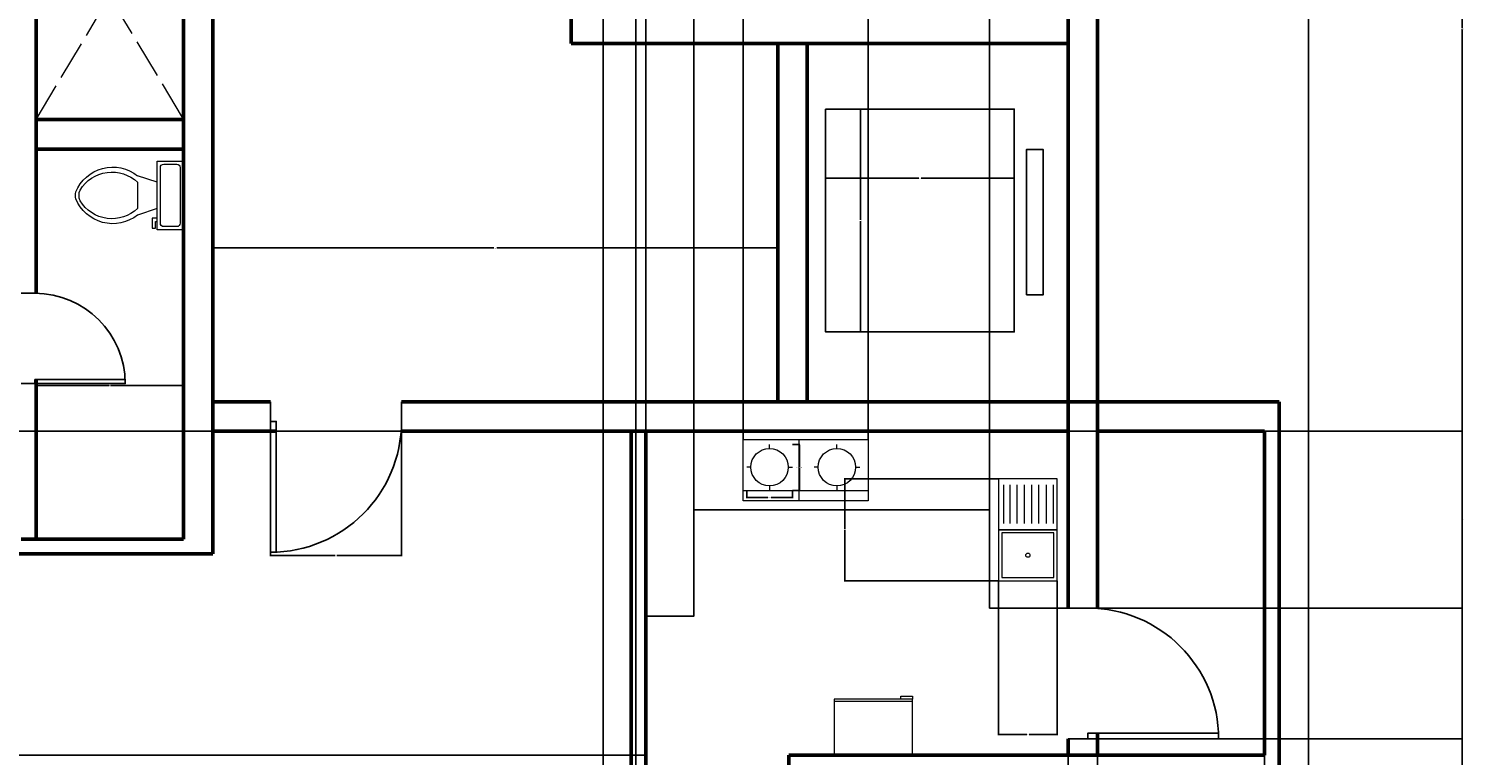
# Model space of a CAD drawing. Units: inches. Extents: x 2032 to 3981, y 840 to 2177.
# Tile 3 of 6: x 2286 to 2725, y 1132 to 1354. Entities that reach past the tile are written whole.
import ezdxf

# ---------------------------------------------------------------- set-up
doc = ezdxf.new("R2010")
doc.units = ezdxf.units.IN
doc.linetypes.add('ACAD_ISO02W100', pattern=[15, 12, -3])
for name, color, linetype, lineweight in [('A-ANNO-DIMS', 2, 'Continuous', 18), ('A-DOOR', 3, 'Continuous', 25), ('A-EQPM', 8, 'Continuous', 18), ('A-FLOR-CASE', 32, 'Continuous', 25), ('A-FLOR-EVTR', 8, 'Continuous', 25), ('A-FLOR-FIXT', 9, 'Continuous', 18), ('A-FLOR-OPEN', 8, 'ACAD_ISO02W100', 13), ('A-WALL', 7, 'Continuous', 50)]:
    doc.layers.add(name, color=color, linetype=linetype, lineweight=lineweight)
doc.styles.get("Standard").update_dxf_attribs({"font": 'arial.ttf'})
doc.dimstyles.get("Standard").update_dxf_attribs({"dimtxt": 0.18, "dimasz": 0.18, "dimexe": 0.18, "dimexo": 0.0625, "dimgap": 0.09, "dimtad": 0, "dimtih": 1, "dimtoh": 1, "dimdec": 4, "dimzin": 0, "dimdsep": 46, "dimtxsty": 'Standard', "dimcen": 0.09, "dimadec": 0, "dimazin": 0, "dimtfac": 1, "dimtdec": 4, "dimtofl": 0, "dimtmove": 0, "dimatfit": 3, "dimfxl": 1, "dimtolj": 1, "dimtzin": 0, "dimarcsym": 0})

# ---------------------------------------------------------------- blocks, each defined once
blk = doc.blocks.new('*U2')
for p, q in [((0, 0), (0, -6)), ((40, 0), (40, -6))]:
    blk.add_line(p, q)
blk.add_lwpolyline([(0, 0), (0, 40), (1.75, 40), (1.75, 0)], close=True)
blk.add_arc((0, 0), 40, 0, 90)
blk = doc.blocks.new('*U4')
for p, q in [((9.5, -6), (9.5, -2)), ((-10, -8.5), (-8, -8.5)), ((-10, -9.5), (-10, -8.5)), ((-8, -8.5), (-8, -8)), ((-7, -8), (-7, -9.5)), ((-4, -8), (-6, -14)), ((4, -8), (6, -14)), ((-7, -9.5), (-10, -9.5)), ((4, -14), (-4, -14))]:
    blk.add_line(p, q)
blk.add_lwpolyline([(10.5, -8), (10.5, 0), (-10.5, 0), (-10.5, -8)], close=True)
for points in [[(-9.5, -2), (-9.5, -6)], [(8.5, -1), (-8.5, -1)], [(-8.5, -7), (8.5, -7)]]:
    blk.add_lwpolyline(points)
for centre, radius, start, end in [((-8.62, -1.88), 0.884, 81.8699, 188.1301), ((8.62, -1.88), 0.884, 351.8699, 98.1301), ((-8.62, -6.12), 0.884, 171.8699, 278.1301), ((8.62, -6.12), 0.884, 261.8699, 8.1301), ((3.52, -21.58), 12.17, 141.4691, 247.9714), ((4.2, -21.82), 11.33, 136.3677, 238.9468), ((-3.52, -21.58), 12.17, 292.0284, 38.5307), ((-4.2, -21.82), 11.33, 301.053, 43.6321), ((0, -27.88), 4, 245.7318, 294.2682), ((0, -29), 4, 254.8605, 285.1395)]:
    blk.add_arc(centre, radius, start, end)
blk = doc.blocks.new('COOKTOP-BURNER')
for p, q in [((6.97, 12.85), (6.97, 14.11)), ((1.25, 7.13), (0, 7.13)), ((12.69, 7.13), (13.97, 7.13)), ((6.97, 1.41), (6.97, 0))]:
    blk.add_line(p, q)
blk.add_circle((6.97, 7.13), 5.72)
blk = doc.blocks.new('*D12')
at = {"layer": 'A-ANNO-DIMS', "color": 0, "lineweight": -2, "transparency": 16777216}
for p, q in [((2519.81, 1226.93), (2522.05, 1226.93)), ((2521.87, 1226.75), (2521.87, 1220.06)), ((2521.87, 1213), (2521.87, 1219.7)), ((2519.81, 1212.82), (2522.05, 1212.82))]:
    blk.add_line(p, q, dxfattribs=at)
at = {"layer": 'A-ANNO-DIMS', "color": 0, "lineweight": 100, "transparency": 16777216}
for points in [[(2521.84, 1226.75), (2521.9, 1226.75), (2521.87, 1226.93)], [(2521.84, 1213), (2521.9, 1213), (2521.87, 1212.82)]]:
    blk.add_solid(points, dxfattribs=at)
at = {"layer": 'Defpoints', "color": 0, "lineweight": 100, "transparency": 16777216}
for p in [(2519.75, 1226.93), (2521.87, 1226.93), (2519.75, 1212.82)]:
    blk.add_point(p, dxfattribs=at)
at = {"layer": 'A-ANNO-DIMS', "color": 0, "transparency": 16777216, "insert": (2521.87, 1219.88), "char_height": 0.18, "attachment_point": 5}
blk.add_mtext('\\A1;BURNER 14 TYP.', dxfattribs=at)
blk = doc.blocks.new('*D13')
at = {"layer": 'A-ANNO-DIMS', "color": 0, "lineweight": -2, "transparency": 16777216}
for p, q in [((2505.78, 1212.76), (2505.78, 1210.53)), ((2505.96, 1210.71), (2512.25, 1210.71)), ((2519.57, 1210.71), (2513.29, 1210.71)), ((2519.75, 1212.76), (2519.75, 1210.53))]:
    blk.add_line(p, q, dxfattribs=at)
at = {"layer": 'A-ANNO-DIMS', "color": 0, "lineweight": 100, "transparency": 16777216}
for points in [[(2505.96, 1210.74), (2505.96, 1210.68), (2505.78, 1210.71)], [(2519.57, 1210.74), (2519.57, 1210.68), (2519.75, 1210.71)]]:
    blk.add_solid(points, dxfattribs=at)
at = {"layer": 'Defpoints', "color": 0, "lineweight": 100, "transparency": 16777216}
for p in [(2505.78, 1212.82), (2519.75, 1212.82), (2519.75, 1210.71)]:
    blk.add_point(p, dxfattribs=at)
at = {"layer": 'A-ANNO-DIMS', "color": 0, "transparency": 16777216, "insert": (2512.77, 1210.71), "char_height": 0.18, "attachment_point": 5}
blk.add_mtext('\\A1;14 TYP.', dxfattribs=at)
blk = doc.blocks.new('*D14')
at = {"layer": 'A-ANNO-DIMS', "color": 0, "lineweight": -2, "transparency": 16777216}
for p, q in [((2078.89, 1518.9), (2078.89, 840.08)), ((2677.35, 1476.9), (2677.35, 840.08)), ((2079.07, 840.26), (2377.73, 840.26)), ((2677.17, 840.26), (2378.52, 840.26))]:
    blk.add_line(p, q, dxfattribs=at)
at = {"layer": 'A-ANNO-DIMS', "color": 0, "lineweight": 100, "transparency": 16777216}
for points in [[(2079.07, 840.29), (2079.07, 840.23), (2078.89, 840.26)], [(2677.17, 840.29), (2677.17, 840.23), (2677.35, 840.26)]]:
    blk.add_solid(points, dxfattribs=at)
at = {"layer": 'Defpoints', "color": 0, "lineweight": 100, "transparency": 16777216}
for p in [(2078.89, 1518.96), (2677.35, 1476.96), (2677.35, 840.26)]:
    blk.add_point(p, dxfattribs=at)
at = {"layer": 'A-ANNO-DIMS', "color": 0, "transparency": 16777216, "insert": (2378.12, 840.26), "char_height": 0.18, "attachment_point": 5}
blk.add_mtext('\\A1;598.5', dxfattribs=at)
blk = doc.blocks.new('*D15')
at = {"layer": 'A-ANNO-DIMS', "color": 0, "lineweight": -2, "transparency": 16777216}
for p, q in [((2456.69, 1820.52), (2724.53, 1820.52)), ((2724.35, 1820.34), (2724.35, 1354.07)), ((2724.35, 887.44), (2724.35, 1353.71)), ((2476.27, 887.26), (2724.53, 887.26))]:
    blk.add_line(p, q, dxfattribs=at)
at = {"layer": 'A-ANNO-DIMS', "color": 0, "lineweight": 100, "transparency": 16777216}
for points in [[(2724.32, 1820.34), (2724.38, 1820.34), (2724.35, 1820.52)], [(2724.32, 887.44), (2724.38, 887.44), (2724.35, 887.26)]]:
    blk.add_solid(points, dxfattribs=at)
at = {"layer": 'Defpoints', "color": 0, "lineweight": 100, "transparency": 16777216}
for p in [(2456.63, 1820.52), (2476.21, 887.26), (2724.35, 887.26)]:
    blk.add_point(p, dxfattribs=at)
at = {"layer": 'A-ANNO-DIMS', "color": 0, "transparency": 16777216, "insert": (2724.35, 1353.89), "char_height": 0.18, "attachment_point": 5}
blk.add_mtext('\\A1;933.3', dxfattribs=at)
blk = doc.blocks.new('*D39')
at = {"layer": 'A-ANNO-DIMS', "color": 0, "lineweight": -2, "transparency": 16777216}
for p, q in [((2288.71, 1198.02), (2288.71, 1245.14)), ((2288.89, 1244.96), (2310.99, 1244.96)), ((2333.53, 1244.96), (2311.43, 1244.96)), ((2333.71, 1198.02), (2333.71, 1245.14))]:
    blk.add_line(p, q, dxfattribs=at)
at = {"layer": 'A-ANNO-DIMS', "color": 0, "lineweight": 100, "transparency": 16777216}
for points in [[(2288.89, 1244.99), (2288.89, 1244.93), (2288.71, 1244.96)], [(2333.53, 1244.99), (2333.53, 1244.93), (2333.71, 1244.96)]]:
    blk.add_solid(points, dxfattribs=at)
at = {"layer": 'Defpoints', "color": 0, "lineweight": 100, "transparency": 16777216}
for p in [(2333.71, 1244.96), (2288.71, 1197.96), (2333.71, 1197.96)]:
    blk.add_point(p, dxfattribs=at)
at = {"layer": 'A-ANNO-DIMS', "color": 0, "transparency": 16777216, "insert": (2311.21, 1244.96), "char_height": 0.18, "attachment_point": 5}
blk.add_mtext('\\A1;45', dxfattribs=at)
blk = doc.blocks.new('*D40')
at = {"layer": 'A-ANNO-DIMS', "color": 0, "lineweight": -2, "transparency": 16777216}
for p, q in [((2342.71, 1240.02), (2342.71, 1287.14)), ((2342.89, 1286.96), (2428.53, 1286.96)), ((2515.07, 1286.96), (2429.43, 1286.96)), ((2515.25, 1240.02), (2515.25, 1287.14))]:
    blk.add_line(p, q, dxfattribs=at)
at = {"layer": 'A-ANNO-DIMS', "color": 0, "lineweight": 100, "transparency": 16777216}
for points in [[(2342.89, 1286.99), (2342.89, 1286.93), (2342.71, 1286.96)], [(2515.07, 1286.99), (2515.07, 1286.93), (2515.25, 1286.96)]]:
    blk.add_solid(points, dxfattribs=at)
at = {"layer": 'Defpoints', "color": 0, "lineweight": 100, "transparency": 16777216}
for p in [(2515.25, 1286.96), (2342.71, 1239.96), (2515.25, 1239.96)]:
    blk.add_point(p, dxfattribs=at)
at = {"layer": 'A-ANNO-DIMS', "color": 0, "transparency": 16777216, "insert": (2428.98, 1286.96), "char_height": 0.18, "attachment_point": 5}
blk.add_mtext('\\A1;172.54', dxfattribs=at)
blk = doc.blocks.new('*D41')
at = {"layer": 'A-ANNO-DIMS', "color": 0, "lineweight": -2, "transparency": 16777216}
for p, q in [((2529.88, 1261.33), (2529.88, 1308.45)), ((2530.06, 1308.27), (2558.31, 1308.27)), ((2587.31, 1308.27), (2559.06, 1308.27)), ((2587.49, 1261.33), (2587.49, 1308.45))]:
    blk.add_line(p, q, dxfattribs=at)
at = {"layer": 'A-ANNO-DIMS', "color": 0, "lineweight": 100, "transparency": 16777216}
for points in [[(2530.06, 1308.3), (2530.06, 1308.24), (2529.88, 1308.27)], [(2587.31, 1308.3), (2587.31, 1308.24), (2587.49, 1308.27)]]:
    blk.add_solid(points, dxfattribs=at)
at = {"layer": 'Defpoints', "color": 0, "lineweight": 100, "transparency": 16777216}
for p in [(2587.49, 1308.27), (2529.88, 1261.27), (2587.49, 1261.27)]:
    blk.add_point(p, dxfattribs=at)
at = {"layer": 'A-ANNO-DIMS', "color": 0, "transparency": 16777216, "insert": (2558.68, 1308.27), "char_height": 0.18, "attachment_point": 5}
blk.add_mtext('\\A1;57.61', dxfattribs=at)
blk = doc.blocks.new('*D42')
at = {"layer": 'A-ANNO-DIMS', "color": 0, "lineweight": -2, "transparency": 16777216}
for p, q in [((2587.42, 1329.38), (2540.31, 1329.38)), ((2540.49, 1329.2), (2540.49, 1295.51)), ((2540.49, 1261.45), (2540.49, 1295.14)), ((2587.42, 1261.27), (2540.31, 1261.27))]:
    blk.add_line(p, q, dxfattribs=at)
at = {"layer": 'A-ANNO-DIMS', "color": 0, "lineweight": 100, "transparency": 16777216}
for points in [[(2540.46, 1329.2), (2540.52, 1329.2), (2540.49, 1329.38)], [(2540.46, 1261.45), (2540.52, 1261.45), (2540.49, 1261.27)]]:
    blk.add_solid(points, dxfattribs=at)
at = {"layer": 'Defpoints', "color": 0, "lineweight": 100, "transparency": 16777216}
for p in [(2540.49, 1329.38), (2587.49, 1329.38), (2587.49, 1261.27)]:
    blk.add_point(p, dxfattribs=at)
at = {"layer": 'A-ANNO-DIMS', "color": 0, "transparency": 16777216, "insert": (2540.49, 1295.33), "char_height": 0.18, "attachment_point": 5}
blk.add_mtext('\\A1;68.11', dxfattribs=at)
blk = doc.blocks.new('*D43')
at = {"layer": 'A-ANNO-DIMS', "color": 0, "lineweight": -2, "transparency": 16777216}
for p, q in [((2360.34, 1239.9), (2360.34, 1192.78)), ((2400.34, 1239.9), (2400.34, 1192.78)), ((2360.52, 1192.96), (2380.11, 1192.96)), ((2400.16, 1192.96), (2380.56, 1192.96))]:
    blk.add_line(p, q, dxfattribs=at)
at = {"layer": 'A-ANNO-DIMS', "color": 0, "lineweight": 100, "transparency": 16777216}
for points in [[(2360.52, 1192.99), (2360.52, 1192.93), (2360.34, 1192.96)], [(2400.16, 1192.99), (2400.16, 1192.93), (2400.34, 1192.96)]]:
    blk.add_solid(points, dxfattribs=at)
at = {"layer": 'Defpoints', "color": 0, "lineweight": 100, "transparency": 16777216}
for p in [(2360.34, 1239.96), (2400.34, 1239.96), (2360.34, 1192.96)]:
    blk.add_point(p, dxfattribs=at)
at = {"layer": 'A-ANNO-DIMS', "color": 0, "transparency": 16777216, "insert": (2380.34, 1192.96), "char_height": 0.18, "attachment_point": 5}
blk.add_mtext('\\A1;40', dxfattribs=at)
blk = doc.blocks.new('*D51')
at = {"layer": 'A-ANNO-DIMS', "color": 0, "lineweight": -2, "transparency": 16777216}
for p, q in [((2474.93, 1231.02), (2474.93, 1867.7)), ((2475.11, 1867.52), (2481.81, 1867.52)), ((2489.42, 1867.52), (2482.72, 1867.52)), ((2489.6, 1231.02), (2489.6, 1867.7))]:
    blk.add_line(p, q, dxfattribs=at)
at = {"layer": 'A-ANNO-DIMS', "color": 0, "lineweight": 100, "transparency": 16777216}
for points in [[(2475.11, 1867.55), (2475.11, 1867.49), (2474.93, 1867.52)], [(2489.42, 1867.55), (2489.42, 1867.49), (2489.6, 1867.52)]]:
    blk.add_solid(points, dxfattribs=at)
at = {"layer": 'Defpoints', "color": 0, "lineweight": 100, "transparency": 16777216}
for p in [(2489.6, 1867.52), (2474.93, 1230.96), (2489.6, 1230.96)]:
    blk.add_point(p, dxfattribs=at)
at = {"layer": 'A-ANNO-DIMS', "color": 0, "transparency": 16777216, "insert": (2482.27, 1867.52), "char_height": 0.18, "attachment_point": 5}
blk.add_mtext('\\A1;14.668', dxfattribs=at)
blk = doc.blocks.new('*D52')
at = {"layer": 'A-ANNO-DIMS', "color": 0, "lineweight": -2, "transparency": 16777216}
for p, q in [((2489.6, 1231.02), (2489.6, 1867.7)), ((2489.78, 1867.52), (2496.71, 1867.52)), ((2504.55, 1867.52), (2497.62, 1867.52)), ((2504.73, 1228.5), (2504.73, 1867.7))]:
    blk.add_line(p, q, dxfattribs=at)
at = {"layer": 'A-ANNO-DIMS', "color": 0, "lineweight": 100, "transparency": 16777216}
for points in [[(2489.78, 1867.55), (2489.78, 1867.49), (2489.6, 1867.52)], [(2504.55, 1867.55), (2504.55, 1867.49), (2504.73, 1867.52)]]:
    blk.add_solid(points, dxfattribs=at)
at = {"layer": 'Defpoints', "color": 0, "lineweight": 100, "transparency": 16777216}
for p in [(2504.73, 1867.52), (2489.6, 1230.96), (2504.73, 1228.44)]:
    blk.add_point(p, dxfattribs=at)
at = {"layer": 'A-ANNO-DIMS', "color": 0, "transparency": 16777216, "insert": (2497.17, 1867.52), "char_height": 0.18, "attachment_point": 5}
blk.add_mtext('\\A1;15.127', dxfattribs=at)
blk = doc.blocks.new('*D53')
at = {"layer": 'A-ANNO-DIMS', "color": 0, "lineweight": -2, "transparency": 16777216}
for p, q in [((2504.73, 1228.5), (2504.73, 1867.7)), ((2504.91, 1867.52), (2523.42, 1867.52)), ((2542.71, 1867.52), (2524.2, 1867.52)), ((2542.89, 1228.5), (2542.89, 1867.7))]:
    blk.add_line(p, q, dxfattribs=at)
at = {"layer": 'A-ANNO-DIMS', "color": 0, "lineweight": 100, "transparency": 16777216}
for points in [[(2504.91, 1867.55), (2504.91, 1867.49), (2504.73, 1867.52)], [(2542.71, 1867.55), (2542.71, 1867.49), (2542.89, 1867.52)]]:
    blk.add_solid(points, dxfattribs=at)
at = {"layer": 'Defpoints', "color": 0, "lineweight": 100, "transparency": 16777216}
for p in [(2542.89, 1867.52), (2504.73, 1228.44), (2542.89, 1228.44)]:
    blk.add_point(p, dxfattribs=at)
at = {"layer": 'A-ANNO-DIMS', "color": 0, "transparency": 16777216, "insert": (2523.81, 1867.52), "char_height": 0.18, "attachment_point": 5}
blk.add_mtext('\\A1;38.16', dxfattribs=at)
blk = doc.blocks.new('*D54')
at = {"layer": 'A-ANNO-DIMS', "color": 0, "lineweight": -2, "transparency": 16777216}
for p, q in [((2542.89, 1228.5), (2542.89, 1867.7)), ((2543.07, 1867.52), (2560.95, 1867.52)), ((2579.75, 1867.52), (2561.88, 1867.52)), ((2579.93, 1207.02), (2579.93, 1867.7))]:
    blk.add_line(p, q, dxfattribs=at)
at = {"layer": 'A-ANNO-DIMS', "color": 0, "lineweight": 100, "transparency": 16777216}
for points in [[(2543.07, 1867.55), (2543.07, 1867.49), (2542.89, 1867.52)], [(2579.75, 1867.55), (2579.75, 1867.49), (2579.93, 1867.52)]]:
    blk.add_solid(points, dxfattribs=at)
at = {"layer": 'Defpoints', "color": 0, "lineweight": 100, "transparency": 16777216}
for p in [(2579.93, 1867.52), (2542.89, 1228.44), (2579.93, 1206.96)]:
    blk.add_point(p, dxfattribs=at)
at = {"layer": 'A-ANNO-DIMS', "color": 0, "transparency": 16777216, "insert": (2561.41, 1867.52), "char_height": 0.18, "attachment_point": 5}
blk.add_mtext('\\A1;37.045', dxfattribs=at)
blk = doc.blocks.new('*D55')
at = {"layer": 'A-ANNO-DIMS', "color": 0, "lineweight": -2, "transparency": 16777216}
for p, q in [((2579.93, 1207.02), (2579.93, 1867.7)), ((2580.11, 1867.52), (2591.71, 1867.52)), ((2603.75, 1867.52), (2592.15, 1867.52)), ((2603.93, 1231.02), (2603.93, 1867.7))]:
    blk.add_line(p, q, dxfattribs=at)
at = {"layer": 'A-ANNO-DIMS', "color": 0, "lineweight": 100, "transparency": 16777216}
for points in [[(2580.11, 1867.55), (2580.11, 1867.49), (2579.93, 1867.52)], [(2603.75, 1867.55), (2603.75, 1867.49), (2603.93, 1867.52)]]:
    blk.add_solid(points, dxfattribs=at)
at = {"layer": 'Defpoints', "color": 0, "lineweight": 100, "transparency": 16777216}
for p in [(2603.93, 1867.52), (2603.93, 1230.96), (2579.93, 1206.96)]:
    blk.add_point(p, dxfattribs=at)
at = {"layer": 'A-ANNO-DIMS', "color": 0, "transparency": 16777216, "insert": (2591.93, 1867.52), "char_height": 0.18, "attachment_point": 5}
blk.add_mtext('\\A1;24', dxfattribs=at)
blk = doc.blocks.new('*D56')
at = {"layer": 'A-ANNO-DIMS', "color": 0, "lineweight": -2, "transparency": 16777216}
for p, q in [((2603.93, 1136.83), (2603.93, 840.08)), ((2474.93, 1131.9), (2474.93, 840.08)), ((2475.11, 840.26), (2539.15, 840.26)), ((2603.75, 840.26), (2539.72, 840.26))]:
    blk.add_line(p, q, dxfattribs=at)
at = {"layer": 'A-ANNO-DIMS', "color": 0, "lineweight": 100, "transparency": 16777216}
for points in [[(2475.11, 840.29), (2475.11, 840.23), (2474.93, 840.26)], [(2603.75, 840.29), (2603.75, 840.23), (2603.93, 840.26)]]:
    blk.add_solid(points, dxfattribs=at)
at = {"layer": 'Defpoints', "color": 0, "lineweight": 100, "transparency": 16777216}
for p in [(2603.93, 1136.9), (2474.93, 1131.96), (2603.93, 840.26)]:
    blk.add_point(p, dxfattribs=at)
at = {"layer": 'A-ANNO-DIMS', "color": 0, "transparency": 16777216, "insert": (2539.43, 840.26), "char_height": 0.18, "attachment_point": 5}
blk.add_mtext('\\A1;129', dxfattribs=at)
blk = doc.blocks.new('*D57')
at = {"layer": 'A-ANNO-DIMS', "color": 0, "lineweight": -2, "transparency": 16777216}
for p, q in [((2612.93, 1138.58), (2612.93, 840.08)), ((2663.93, 1131.9), (2663.93, 840.08)), ((2613.11, 840.26), (2638.23, 840.26)), ((2663.75, 840.26), (2638.64, 840.26))]:
    blk.add_line(p, q, dxfattribs=at)
at = {"layer": 'A-ANNO-DIMS', "color": 0, "lineweight": 100, "transparency": 16777216}
for points in [[(2613.11, 840.29), (2613.11, 840.23), (2612.93, 840.26)], [(2663.75, 840.29), (2663.75, 840.23), (2663.93, 840.26)]]:
    blk.add_solid(points, dxfattribs=at)
at = {"layer": 'Defpoints', "color": 0, "lineweight": 100, "transparency": 16777216}
for p in [(2612.93, 1138.65), (2663.93, 1131.96), (2663.93, 840.26)]:
    blk.add_point(p, dxfattribs=at)
at = {"layer": 'A-ANNO-DIMS', "color": 0, "transparency": 16777216, "insert": (2638.43, 840.26), "char_height": 0.18, "attachment_point": 5}
blk.add_mtext('\\A1;51', dxfattribs=at)
blk = doc.blocks.new('*D58')
at = {"layer": 'A-ANNO-DIMS', "color": 0, "lineweight": -2, "transparency": 16777216}
for p, q in [((2474.87, 1230.96), (2031.71, 1230.96)), ((2031.89, 1230.78), (2031.89, 1181.64)), ((2031.89, 1132.14), (2031.89, 1181.28)), ((2474.87, 1131.96), (2031.71, 1131.96))]:
    blk.add_line(p, q, dxfattribs=at)
at = {"layer": 'A-ANNO-DIMS', "color": 0, "lineweight": 100, "transparency": 16777216}
for points in [[(2031.86, 1230.78), (2031.92, 1230.78), (2031.89, 1230.96)], [(2031.86, 1132.14), (2031.92, 1132.14), (2031.89, 1131.96)]]:
    blk.add_solid(points, dxfattribs=at)
at = {"layer": 'Defpoints', "color": 0, "lineweight": 100, "transparency": 16777216}
for p in [(2474.93, 1230.96), (2031.89, 1131.96), (2474.93, 1131.96)]:
    blk.add_point(p, dxfattribs=at)
at = {"layer": 'A-ANNO-DIMS', "color": 0, "transparency": 16777216, "insert": (2031.89, 1181.46), "char_height": 0.18, "attachment_point": 5}
blk.add_mtext('\\A1;99', dxfattribs=at)
blk = doc.blocks.new('*D59')
at = {"layer": 'A-ANNO-DIMS', "color": 0, "lineweight": -2, "transparency": 16777216}
for p, q in [((2604, 1176.9), (2724.53, 1176.9)), ((2724.35, 1176.72), (2724.35, 1157.08)), ((2724.35, 1137.08), (2724.35, 1156.71)), ((2604, 1136.9), (2724.53, 1136.9))]:
    blk.add_line(p, q, dxfattribs=at)
at = {"layer": 'A-ANNO-DIMS', "color": 0, "lineweight": 100, "transparency": 16777216}
for points in [[(2724.32, 1176.72), (2724.38, 1176.72), (2724.35, 1176.9)], [(2724.32, 1137.08), (2724.38, 1137.08), (2724.35, 1136.9)]]:
    blk.add_solid(points, dxfattribs=at)
at = {"layer": 'Defpoints', "color": 0, "lineweight": 100, "transparency": 16777216}
for p in [(2603.93, 1176.9), (2603.93, 1136.9), (2724.35, 1136.9)]:
    blk.add_point(p, dxfattribs=at)
at = {"layer": 'A-ANNO-DIMS', "color": 0, "transparency": 16777216, "insert": (2724.35, 1156.9), "char_height": 0.18, "attachment_point": 5}
blk.add_mtext('\\A1;40', dxfattribs=at)
blk = doc.blocks.new('*D60')
at = {"layer": 'A-ANNO-DIMS', "color": 0, "lineweight": -2, "transparency": 16777216}
for p, q in [((2604, 1230.96), (2724.53, 1230.96)), ((2724.35, 1230.78), (2724.35, 1204.11)), ((2724.35, 1177.08), (2724.35, 1203.75)), ((2604, 1176.9), (2724.53, 1176.9))]:
    blk.add_line(p, q, dxfattribs=at)
at = {"layer": 'A-ANNO-DIMS', "color": 0, "lineweight": 100, "transparency": 16777216}
for points in [[(2724.32, 1230.78), (2724.38, 1230.78), (2724.35, 1230.96)], [(2724.32, 1177.08), (2724.38, 1177.08), (2724.35, 1176.9)]]:
    blk.add_solid(points, dxfattribs=at)
at = {"layer": 'Defpoints', "color": 0, "lineweight": 100, "transparency": 16777216}
for p in [(2603.93, 1230.96), (2603.93, 1176.9), (2724.35, 1176.9)]:
    blk.add_point(p, dxfattribs=at)
at = {"layer": 'A-ANNO-DIMS', "color": 0, "transparency": 16777216, "insert": (2724.35, 1203.93), "char_height": 0.18, "attachment_point": 5}
blk.add_mtext('\\A1;54.06', dxfattribs=at)
blk = doc.blocks.new('*D61')
at = {"layer": 'A-ANNO-DIMS', "color": 0, "lineweight": -2, "transparency": 16777216}
for p, q in [((2582.64, 1216.44), (2535.52, 1216.44)), ((2535.7, 1216.26), (2535.7, 1201.03)), ((2535.7, 1185.43), (2535.7, 1200.67)), ((2582.64, 1185.25), (2535.52, 1185.25))]:
    blk.add_line(p, q, dxfattribs=at)
at = {"layer": 'A-ANNO-DIMS', "color": 0, "lineweight": 100, "transparency": 16777216}
for points in [[(2535.67, 1216.26), (2535.73, 1216.26), (2535.7, 1216.44)], [(2535.67, 1185.43), (2535.73, 1185.43), (2535.7, 1185.25)]]:
    blk.add_solid(points, dxfattribs=at)
at = {"layer": 'Defpoints', "color": 0, "lineweight": 100, "transparency": 16777216}
for p in [(2535.7, 1216.44), (2582.7, 1216.44), (2582.7, 1185.25)]:
    blk.add_point(p, dxfattribs=at)
at = {"layer": 'A-ANNO-DIMS', "color": 0, "transparency": 16777216, "insert": (2535.7, 1200.85), "char_height": 0.18, "attachment_point": 5}
blk.add_mtext('\\A1;31.19', dxfattribs=at)
blk = doc.blocks.new('*D62')
at = {"layer": 'A-ANNO-DIMS', "color": 0, "lineweight": -2, "transparency": 16777216}
for p, q in [((2582.7, 1185.19), (2582.7, 1138.07)), ((2600.61, 1185.19), (2600.61, 1138.07)), ((2582.88, 1138.25), (2591.29, 1138.25)), ((2600.43, 1138.25), (2592.03, 1138.25))]:
    blk.add_line(p, q, dxfattribs=at)
at = {"layer": 'A-ANNO-DIMS', "color": 0, "lineweight": 100, "transparency": 16777216}
for points in [[(2582.88, 1138.28), (2582.88, 1138.22), (2582.7, 1138.25)], [(2600.43, 1138.28), (2600.43, 1138.22), (2600.61, 1138.25)]]:
    blk.add_solid(points, dxfattribs=at)
at = {"layer": 'Defpoints', "color": 0, "lineweight": 100, "transparency": 16777216}
for p in [(2582.7, 1185.25), (2600.61, 1185.25), (2582.7, 1138.25)]:
    blk.add_point(p, dxfattribs=at)
at = {"layer": 'A-ANNO-DIMS', "color": 0, "transparency": 16777216, "insert": (2591.66, 1138.25), "char_height": 0.18, "attachment_point": 5}
blk.add_mtext('\\A1;17.91', dxfattribs=at)
blk = doc.blocks.new('*D65')
at = {"layer": 'A-ANNO-DIMS', "color": 0, "lineweight": -2, "transparency": 16777216}
for p, q in [((2461.93, 1358.4), (2461.93, 840.08)), ((2471.93, 1358.4), (2471.93, 840.08)), ((2462.11, 840.26), (2466.72, 840.26)), ((2471.75, 840.26), (2467.14, 840.26))]:
    blk.add_line(p, q, dxfattribs=at)
at = {"layer": 'A-ANNO-DIMS', "color": 0, "lineweight": 100, "transparency": 16777216}
for points in [[(2462.11, 840.29), (2462.11, 840.23), (2461.93, 840.26)], [(2471.75, 840.29), (2471.75, 840.23), (2471.93, 840.26)]]:
    blk.add_solid(points, dxfattribs=at)
at = {"layer": 'Defpoints', "color": 0, "lineweight": 100, "transparency": 16777216}
for p in [(2461.93, 1358.46), (2471.93, 1358.46), (2471.93, 840.26)]:
    blk.add_point(p, dxfattribs=at)
at = {"layer": 'A-ANNO-DIMS', "color": 0, "transparency": 16777216, "insert": (2466.93, 840.26), "char_height": 0.18, "attachment_point": 5}
blk.add_mtext('\\A1;10', dxfattribs=at)

msp = doc.modelspace()

# ---------------------------------------------------------------- linework, layer by layer
at = {"layer": 'A-EQPM'}
for p, q in [((2521.7978, 1209.697), (2521.7978, 1228.4424)), ((2504.7296, 1212.8236), (2542.8893, 1212.8236)), ((2532.4941, 1148.4696), (2556.4041, 1148.4696))]:
    msp.add_line(p, q, dxfattribs=at)
for points in [[(2504.7296, 1228.4424), (2542.8893, 1228.4424), (2542.8893, 1209.697), (2504.7296, 1209.697)], [(2532.4941, 1131.9584), (2556.4041, 1131.9584), (2556.4041, 1149.0406), (2532.4941, 1149.0406)], [(2556.4041, 1149.0406), (2552.8315, 1149.0406), (2552.8315, 1150.0096), (2556.4041, 1150.0096)]]:
    msp.add_lwpolyline(points, close=True, dxfattribs=at)
at = {"layer": 'A-FLOR-CASE'}
for p, q in [((2489.6025, 1230.9584), (2489.6025, 1206.9584)), ((2489.6025, 1206.9584), (2579.9346, 1206.9584)), ((2579.9346, 1176.8961), (2579.9346, 1206.9584)), ((2603.9346, 1176.8961), (2579.9346, 1176.8961))]:
    msp.add_line(p, q, dxfattribs=at)
msp.add_lwpolyline([(2474.9346, 1230.9584), (2489.6025, 1230.9584), (2489.6025, 1174.4121), (2474.9346, 1174.4121)], close=True, dxfattribs=at)
at = {"layer": 'A-FLOR-EVTR'}
for points in [[(2529.8789, 1329.3824), (2587.4861, 1329.3824), (2587.4861, 1261.2693), (2529.8789, 1261.2693)], [(2591.2595, 1272.5796), (2596.2907, 1272.5796), (2596.2907, 1317.0667), (2591.2595, 1317.0667)]]:
    msp.add_lwpolyline(points, close=True, dxfattribs=at)
at = {"layer": 'A-FLOR-FIXT'}
for p, q in [((2584.2758, 1202.7191), (2584.2758, 1214.5467)), ((2586.2164, 1202.7191), (2586.2164, 1214.5467)), ((2588.3511, 1202.7191), (2588.3511, 1214.5467)), ((2590.6152, 1202.7191), (2590.6152, 1214.5467)), ((2592.8793, 1202.7191), (2592.8793, 1214.5467)), ((2595.014, 1202.7191), (2595.014, 1214.5467)), ((2597.3428, 1202.7191), (2597.3428, 1214.5467)), ((2599.4775, 1202.7191), (2599.4775, 1214.5467)), ((2582.7035, 1200.8473), (2600.6134, 1200.8473))]:
    msp.add_line(p, q, dxfattribs=at)
for points in [[(2582.7035, 1185.2514), (2600.6134, 1185.2514), (2600.6134, 1216.4432), (2582.7035, 1216.4432)], [(2582.7035, 1185.2514), (2600.6134, 1185.2514), (2600.6134, 1200.8473), (2582.7035, 1200.8473)], [(2583.7035, 1186.2514), (2599.6134, 1186.2514), (2599.6134, 1199.8473), (2583.7035, 1199.8473)]]:
    msp.add_lwpolyline(points, close=True, dxfattribs=at)
msp.add_circle((2591.6585, 1193.0493), 0.6386, dxfattribs=at)
at = {"layer": 'A-FLOR-OPEN'}
for p, q in [((2288.7092, 1326.1705), (2333.7092, 1401.441)), ((2288.7092, 1401.441), (2333.7092, 1326.1705))]:
    msp.add_line(p, q, dxfattribs=at)
at = {"layer": 'A-WALL'}
for p, q in [((2333.7092, 1293.9584), (2333.7092, 1518.9584)), ((2342.7092, 1302.9584), (2342.7092, 1518.9584)), ((2603.9346, 1239.9584), (2603.9346, 1476.9584)), ((2612.9346, 1230.9584), (2612.9346, 1476.9584)), ((2288.7092, 1353.9584), (2288.7092, 1452.8709)), ((2452.1278, 1349.4584), (2452.1278, 1358.4584)), ((2288.7092, 1273.096), (2288.7092, 1353.9584)), ((2603.9346, 1349.4584), (2452.1278, 1349.4584)), ((2515.2511, 1239.9584), (2515.2511, 1349.4584)), ((2524.2511, 1239.9584), (2524.2511, 1349.4584)), ((2333.7092, 1326.1705), (2288.7092, 1326.1705)), ((2333.7092, 1317.1705), (2288.7092, 1317.1705)), ((2342.7092, 1193.4584), (2342.7092, 1302.9584)), ((2333.7092, 1197.9584), (2333.7092, 1293.9584)), ((2288.7092, 1197.9584), (2288.7092, 1246.7207)), ((2360.3352, 1239.9584), (2342.7092, 1239.9584)), ((2470.4346, 1239.9584), (2400.3352, 1239.9584)), ((2470.4346, 1239.9584), (2603.9346, 1239.9584)), ((2543.9346, 1239.9584), (2515.2511, 1239.9584)), ((2603.9346, 1239.9584), (2543.9346, 1239.9584)), ((2603.9346, 1239.9584), (2603.9346, 1176.8961)), ((2668.4346, 1239.9584), (2603.9346, 1239.9584)), ((2668.4346, 1127.4584), (2668.4346, 1239.9584)), ((2362.0852, 1230.9584), (2342.7092, 1230.9584)), ((2474.9346, 1230.9584), (2400.2226, 1230.9584)), ((2470.4346, 1127.4584), (2470.4346, 1230.9584)), ((2474.9346, 1131.9584), (2474.9346, 1230.9584)), ((2474.9346, 1230.9584), (2603.9346, 1230.9584)), ((2663.9346, 1230.9584), (2612.9346, 1230.9584)), ((2612.9346, 1230.9584), (2612.9346, 1176.7834)), ((2663.9346, 1131.9584), (2663.9346, 1230.9584)), ((2663.9346, 1131.9584), (2663.9346, 1230.9584)), ((2284.2092, 1197.9584), (2288.7092, 1197.9584)), ((2288.7092, 1197.9584), (2333.7092, 1197.9584)), ((2276.813, 1193.4584), (2288.7092, 1193.4584)), ((2342.7092, 1193.4584), (2288.7092, 1193.4584)), ((2288.7092, 1193.4584), (2342.7092, 1193.4584)), ((2603.9346, 1136.8961), (2603.9346, 1131.9584)), ((2612.9346, 1138.6461), (2612.9346, 1131.9584)), ((2474.9346, 1131.9584), (2475.0017, 1127.4584)), ((2603.9346, 1131.9584), (2518.6525, 1131.9584)), ((2518.6525, 1127.4584), (2518.6525, 1131.9584)), ((2522.7092, 1131.9584), (2641.2092, 1131.9584)), ((2641.2092, 1131.9584), (2663.9346, 1131.9584))]:
    msp.add_line(p, q, dxfattribs=at)

# ---------------------------------------------------------------- block references
at = {"layer": 'A-DOOR', "xscale": -0.6896122567198519, "yscale": 0.6896122567198519, "zscale": 0.6896122567198519, "rotation": 270}
msp.add_blockref('*U2', (2288.3469, 1245.5139), dxfattribs=at)
at = {"layer": 'A-DOOR', "xscale": -1}
for p, rotation in [((2360.3352, 1233.9584), 180), ((2609.9346, 1136.8961), 270)]:
    msp.add_blockref('*U2', p, dxfattribs=dict(at, rotation=rotation))
at = {"layer": 'A-EQPM'}
for p in [(2505.783, 1212.824), (2526.3496, 1212.824)]:
    msp.add_blockref('COOKTOP-BURNER', p, dxfattribs=at)
at = {"layer": 'A-FLOR-FIXT', "xscale": -1, "rotation": 270}
msp.add_blockref('*U4', (2333.7092, 1303.0134), dxfattribs=at)

# ---------------------------------------------------------------- dimensions: what is measured, and where the dimension line sits
at = {"layer": 'A-ANNO-DIMS'}
for base, p1, p2, override, picture, middle in [((2489.6025, 1867.5217), (2474.9346, 1230.9584), (2489.6025, 1230.9584), {"dimdec": 3, "dimlfac": 1, "dimrnd": 0, "dimzin": 0, "dimdsep": 46, "dimlunit": 2}, '*D51', (2482.2686, 1867.5217)), ((2504.7296, 1867.5217), (2489.6025, 1230.9584), (2504.7296, 1228.4424), {"dimdec": 3, "dimlfac": 1, "dimrnd": 0, "dimzin": 0, "dimdsep": 46, "dimlunit": 2}, '*D52', (2497.1661, 1867.5217)), ((2542.8893, 1867.5217), (2504.7296, 1228.4424), (2542.8893, 1228.4424), {"dimdec": 2, "dimlfac": 1, "dimrnd": 0, "dimzin": 0, "dimdsep": 46, "dimlunit": 2}, '*D53', (2523.8094, 1867.5217)), ((2579.9346, 1867.5217), (2542.8893, 1228.4424), (2579.9346, 1206.9584), {"dimdec": 3, "dimlfac": 1, "dimrnd": 0, "dimzin": 0, "dimdsep": 46, "dimlunit": 2}, '*D54', (2561.412, 1867.5217)), ((2603.9346, 1867.5217), (2579.9346, 1206.9584), (2603.9346, 1230.9584), {"dimdec": 0, "dimlfac": 1, "dimrnd": 0, "dimzin": 0, "dimdsep": 46, "dimlunit": 2}, '*D55', (2591.9346, 1867.5217)), ((2677.3537, 840.2551), (2078.8911, 1518.9584), (2677.3537, 1476.9584), {"dimdec": 1, "dimlfac": 1, "dimrnd": 0, "dimzin": 0, "dimdsep": 46, "dimlunit": 2}, '*D14', (2378.1224, 840.2551)), ((2471.9346, 840.2551), (2461.9346, 1358.4584), (2471.9346, 1358.4584), {"dimdec": 0, "dimlfac": 1, "dimrnd": 0, "dimzin": 0, "dimdsep": 46, "dimlunit": 2}, '*D65', (2466.9346, 840.2551)), ((2587.4861, 1308.2693), (2529.8789, 1261.2693), (2587.4861, 1261.2693), {"dimdec": 2, "dimlfac": 1, "dimrnd": 0, "dimzin": 0, "dimdsep": 46, "dimlunit": 2}, '*D41', (2558.6825, 1308.2693)), ((2515.2511, 1286.9584), (2342.7092, 1239.9584), (2515.2511, 1239.9584), {"dimdec": 2, "dimlfac": 1, "dimrnd": 0, "dimzin": 0, "dimdsep": 46, "dimlunit": 2}, '*D40', (2428.9802, 1286.9584)), ((2333.7092, 1244.9584), (2288.7092, 1197.9584), (2333.7092, 1197.9584), {"dimdec": 0, "dimlfac": 1, "dimrnd": 0, "dimzin": 0, "dimdsep": 46, "dimlunit": 2}, '*D39', (2311.2092, 1244.9584)), ((2603.9346, 840.2551), (2474.9346, 1131.9584), (2603.9346, 1136.8961), {"dimdec": 0, "dimlfac": 1, "dimrnd": 0, "dimzin": 0, "dimdsep": 46, "dimlunit": 2}, '*D56', (2539.4346, 840.2551)), ((2663.9346, 840.2551), (2612.9346, 1138.6461), (2663.9346, 1131.9584), {"dimdec": 0, "dimlfac": 1, "dimrnd": 0, "dimzin": 0, "dimdsep": 46, "dimlunit": 2}, '*D57', (2638.4346, 840.2551))]:
    dim = msp.add_linear_dim(base=base, p1=p1, p2=p2, dimstyle='Standard', override=override, dxfattribs=at)
    dim.commit()
    dim.dimension.update_dxf_attribs({"geometry": picture, "text_midpoint": middle})
for base, p1, p2, angle, override, picture, middle in [((2724.3537, 887.2551), (2456.6278, 1820.5217), (2476.2092, 887.2551), 90, {"dimdec": 1, "dimlfac": 1, "dimrnd": 0, "dimzin": 0, "dimdsep": 46, "dimlunit": 2}, '*D15', (2724.3537, 1353.8884)), ((2540.4861, 1329.3824), (2587.4861, 1261.2693), (2587.4861, 1329.3824), 90, {"dimdec": 2, "dimlfac": 1, "dimrnd": 0, "dimzin": 0, "dimdsep": 46, "dimlunit": 2}, '*D42', (2540.4861, 1295.3258)), ((2360.3352, 1192.9584), (2400.3352, 1239.9584), (2360.3352, 1239.9584), 180, {"dimdec": 0, "dimlfac": 1, "dimrnd": 0, "dimzin": 0, "dimdsep": 46, "dimlunit": 2}, '*D43', (2380.3352, 1192.9584)), ((2031.8911, 1131.9584), (2474.9346, 1230.9584), (2474.9346, 1131.9584), 90, {"dimdec": 0, "dimlfac": 1, "dimrnd": 0, "dimzin": 0, "dimdsep": 46, "dimlunit": 2}, '*D58', (2031.8911, 1181.4584)), ((2724.3537, 1176.8961), (2603.9346, 1230.9584), (2603.9346, 1176.8961), 90, {"dimdec": 2, "dimlfac": 1, "dimrnd": 0, "dimzin": 0, "dimdsep": 46, "dimlunit": 2}, '*D60', (2724.3537, 1203.9273)), ((2535.7035, 1216.4432), (2582.7035, 1185.2514), (2582.7035, 1216.4432), 90, {"dimdec": 2, "dimlfac": 1, "dimrnd": 0, "dimzin": 0, "dimdsep": 46, "dimlunit": 2}, '*D61', (2535.7035, 1200.8473)), ((2582.7035, 1138.2514), (2600.6134, 1185.2514), (2582.7035, 1185.2514), 180, {"dimdec": 2, "dimlfac": 1, "dimrnd": 0, "dimzin": 0, "dimdsep": 46, "dimlunit": 2}, '*D62', (2591.6585, 1138.2514)), ((2724.3537, 1136.8961), (2603.9346, 1176.8961), (2603.9346, 1136.8961), 90, {"dimdec": 0, "dimlfac": 1, "dimrnd": 0, "dimzin": 0, "dimdsep": 46, "dimlunit": 2}, '*D59', (2724.3537, 1156.8961))]:
    dim = msp.add_linear_dim(base=base, p1=p1, p2=p2, angle=angle, dimstyle='Standard', override=override, dxfattribs=at)
    dim.commit()
    dim.dimension.update_dxf_attribs({"geometry": picture, "text_midpoint": middle})
dim = msp.add_linear_dim(base=(2521.8652, 1226.9303), p1=(2519.7492, 1212.8236), p2=(2519.7492, 1226.9303), angle=90, text='BURNER <> TYP.', dimstyle='Standard', override={"dimdec": 0, "dimlfac": 1, "dimrnd": 0, "dimzin": 0, "dimdsep": 46, "dimlunit": 2}, dxfattribs=at)
dim.commit()
dim.dimension.update_dxf_attribs({"geometry": '*D12', "text_midpoint": (2521.8652, 1219.8769)})
dim = msp.add_linear_dim(base=(2519.7492, 1210.7075), p1=(2505.783, 1212.8236), p2=(2519.7492, 1212.8236), text='<> TYP.', dimstyle='Standard', override={"dimdec": 0, "dimlfac": 1, "dimrnd": 0, "dimzin": 0, "dimdsep": 46, "dimlunit": 2}, dxfattribs=at)
dim.commit()
dim.dimension.update_dxf_attribs({"geometry": '*D13', "text_midpoint": (2512.7661, 1210.7075)})

doc.saveas('drawing.dxf')
